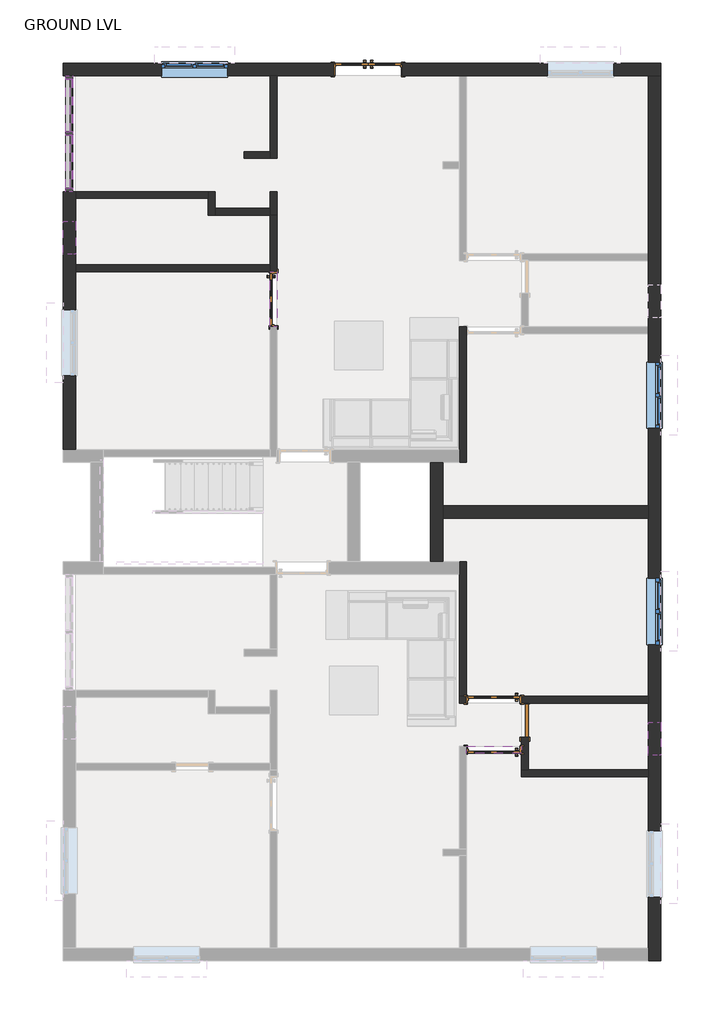
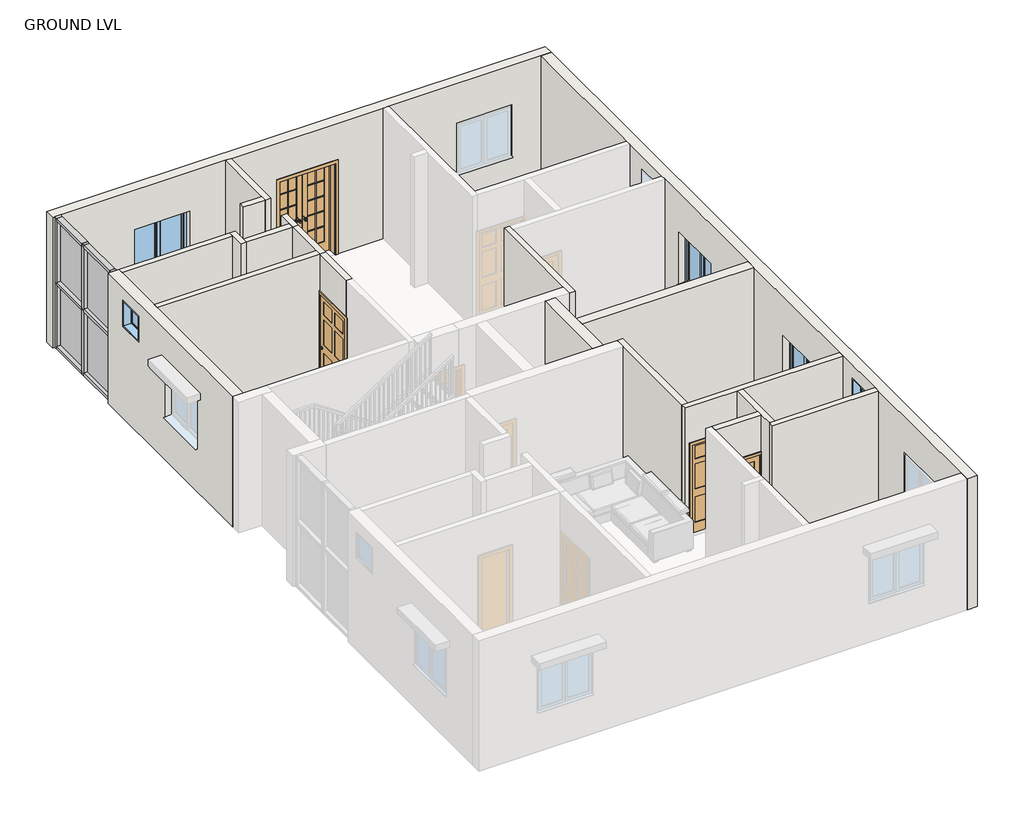
# One storey, part 2 of 4: 20 walls, 12 members, 5 doors, 5 windows, 4 plates.
"""IFC4 building model written with IfcOpenShell, lengths in millimetres."""

from ifc_helpers import new_model, si_unit, frame, origin, place, context, project, spatial, polyline, outline, extrude, faceted_brep, transform, mapped, element, save
from components import door_interior_double_full_glass_wood_4_x_7_exterior_door_6b6f14de, door_6a452240, door_3d68aebc, single_flush_flush_door_2_x_7_931cabab, member_801a2072, member_82905deb, member_88aa5c81, member_4491d118, system_panel_glazed_a8655be6, window_80340324, w2_windows_4_x_4_9dec5fc7

model = new_model("IFC4")

# Units and contexts
model_context = context("Model", 3, world=origin())
ifc_project = project(units=[si_unit("LENGTHUNIT", "METRE", prefix="MILLI")], contexts=[model_context])

# Site, building, storey
site = spatial("IfcSite", under=ifc_project)
building = spatial("IfcBuilding", under=site)
storey = spatial("IfcBuildingStorey", under=building, Name="GROUND LVL", Elevation=3048.0)

# Doors
placement = place(None, origin())
door_interior_double_full_glass_wood_4_x_7_exterior_door_shape = door_interior_double_full_glass_wood_4_x_7_exterior_door_6b6f14de(model_context)
element("IfcDoor", 1, ObjectType="Door-Interior-Double-Full Glass-Wood : 4' x 7' exterior door", at=placement, inside=storey, context=model_context, shape_type="MappedRepresentation", body=[
    mapped(door_interior_double_full_glass_wood_4_x_7_exterior_door_shape, transform((-817.6012202, 13160.1059003, 3048.0), x_axis=(1.0, 0.0, 0.0), y_axis=(0.0, 1.0, 0.0), z_axis=(0.0, 0.0, 1.0))),
])
door_shape = door_6a452240(model_context)
element("IfcDoor", 2, ObjectType="Door-Interior-Single-6_Panel-Wood : interior door 3' 4\" x 7'", at=placement, inside=storey, context=model_context, shape_type="MappedRepresentation", body=[
    mapped(door_shape, transform((-2560.6762202, 8927.8309003, 3048.0), x_axis=(0.0, -1.0, 0.0), y_axis=(1.0, 0.0, 0.0), z_axis=(0.0, 0.0, 1.0))),
])
element("IfcDoor", 3, ObjectType="Door-Interior-Single-6_Panel-Wood : interior door 3' 4\" x 7'", at=placement, inside=storey, context=model_context, shape_type="MappedRepresentation", body=[
    mapped(door_shape, transform((1493.7987798, 1565.0059003, 3048.0), x_axis=(-1.0, 0.0, 0.0), y_axis=(0.0, -1.0, 0.0), z_axis=(0.0, 0.0, 1.0))),
])
door_2_shape = door_3d68aebc(model_context)
element("IfcDoor", 4, ObjectType="Door-Interior-Single-6_Panel-Wood : interior door 3' 4\" x 7'", at=placement, inside=storey, context=model_context, shape_type="MappedRepresentation", body=[
    mapped(door_2_shape, transform((1493.7987798, 644.2559003, 3048.0), x_axis=(-1.0, 0.0, 0.0), y_axis=(0.0, -1.0, 0.0), z_axis=(0.0, 0.0, 1.0))),
])
single_flush_flush_door_2_x_7_shape = single_flush_flush_door_2_x_7_931cabab(model_context)
element("IfcDoor", 5, ObjectType="Single-Flush : flush door 2' x 7'", at=placement, inside=storey, context=model_context, shape_type="MappedRepresentation", body=[
    mapped(single_flush_flush_door_2_x_7_shape, transform((2065.2987798, 1180.8309003, 3048.0), x_axis=(0.0, 1.0, 0.0), y_axis=(-1.0, 0.0, 0.0), z_axis=(0.0, 0.0, 1.0))),
])

# Members
member_shape = member_801a2072(model_context)
element("IfcMember", 6, ObjectType="Rectangular Mullion : 2.5\" x 5\" rectangular", at=placement, inside=storey, context=model_context, shape_type="MappedRepresentation", body=[
    mapped(member_shape, transform((-6316.7012202, 10972.5309003, 6096.0), x_axis=(0.0, 0.0, 1.0), y_axis=(-1.0, 0.0, 0.0), z_axis=(0.0, -1.0, 0.0))),
])
element("IfcMember", 7, ObjectType="Rectangular Mullion : 2.5\" x 5\" rectangular", at=placement, inside=storey, context=model_context, shape_type="MappedRepresentation", body=[
    mapped(member_shape, transform((-6316.7012202, 12007.5809003, 6096.0), x_axis=(0.0, 0.0, 1.0), y_axis=(-1.0, 0.0, 0.0), z_axis=(0.0, -1.0, 0.0))),
])
element("IfcMember", 8, ObjectType="Rectangular Mullion : 2.5\" x 5\" rectangular", at=placement, inside=storey, context=model_context, shape_type="MappedRepresentation", body=[
    mapped(member_shape, transform((-6316.7012202, 12979.1309003, 3048.0), x_axis=(0.0, 0.0, -1.0), y_axis=(-1.0, 0.0, 0.0), z_axis=(0.0, 1.0, 0.0))),
])
element("IfcMember", 9, ObjectType="Rectangular Mullion : 2.5\" x 5\" rectangular", at=placement, inside=storey, context=model_context, shape_type="MappedRepresentation", body=[
    mapped(member_shape, transform((-6316.7012202, 11944.0809003, 3048.0), x_axis=(0.0, 0.0, -1.0), y_axis=(-1.0, 0.0, 0.0), z_axis=(0.0, 1.0, 0.0))),
])
member_2_shape = member_82905deb(model_context)
element("IfcMember", 10, ObjectType="Rectangular Mullion : 2.5\" x 5\" rectangular", at=placement, inside=storey, context=model_context, shape_type="MappedRepresentation", body=[
    mapped(member_2_shape, transform((-6316.7012202, 11975.8309003, 3048.0), x_axis=(0.0, -1.0, 0.0), y_axis=(-1.0, 0.0, 0.0), z_axis=(0.0, 0.0, -1.0))),
])
member_3_shape = member_88aa5c81(model_context)
element("IfcMember", 11, ObjectType="Rectangular Mullion : 2.5\" x 5\" rectangular", at=placement, inside=storey, context=model_context, shape_type="MappedRepresentation", body=[
    mapped(member_3_shape, transform((-6316.7012202, 12007.5809003, 4572.0), x_axis=(0.0, 0.0, 1.0), y_axis=(-1.0, 0.0, 0.0), z_axis=(0.0, -1.0, 0.0))),
])
element("IfcMember", 12, ObjectType="Rectangular Mullion : 2.5\" x 5\" rectangular", at=placement, inside=storey, context=model_context, shape_type="MappedRepresentation", body=[
    mapped(member_3_shape, transform((-6316.7012202, 10972.5309003, 4572.0), x_axis=(0.0, 0.0, 1.0), y_axis=(-1.0, 0.0, 0.0), z_axis=(0.0, -1.0, 0.0))),
])
element("IfcMember", 13, ObjectType="Rectangular Mullion : 2.5\" x 5\" rectangular", at=placement, inside=storey, context=model_context, shape_type="MappedRepresentation", body=[
    mapped(member_2_shape, transform((-6316.7012202, 11975.8309003, 4572.0), x_axis=(0.0, -1.0, 0.0), y_axis=(-1.0, 0.0, 0.0), z_axis=(0.0, 0.0, -1.0))),
])
member_4_shape = member_4491d118(model_context)
element("IfcMember", 14, ObjectType="Rectangular Mullion : 2.5\" x 5\" rectangular", at=placement, inside=storey, context=model_context, shape_type="MappedRepresentation", body=[
    mapped(member_4_shape, transform((-6316.7012202, 10909.0309003, 3048.0), x_axis=(0.0, -1.0, 0.0), y_axis=(-1.0, 0.0, 0.0), z_axis=(0.0, 0.0, -1.0))),
])
element("IfcMember", 15, ObjectType="Rectangular Mullion : 2.5\" x 5\" rectangular", at=placement, inside=storey, context=model_context, shape_type="MappedRepresentation", body=[
    mapped(member_4_shape, transform((-6316.7012202, 13042.6309003, 6096.0), x_axis=(0.0, 1.0, 0.0), y_axis=(-1.0, 0.0, 0.0), z_axis=(0.0, 0.0, 1.0))),
])
element("IfcMember", 16, ObjectType="Rectangular Mullion : 2.5\" x 5\" rectangular", at=placement, inside=storey, context=model_context, shape_type="MappedRepresentation", body=[
    mapped(member_4_shape, transform((-6316.7012202, 10909.0309003, 4572.0), x_axis=(0.0, -1.0, 0.0), y_axis=(-1.0, 0.0, 0.0), z_axis=(0.0, 0.0, -1.0))),
])
element("IfcMember", 17, ObjectType="Rectangular Mullion : 2.5\" x 5\" rectangular", at=placement, inside=storey, context=model_context, shape_type="MappedRepresentation", body=[
    mapped(member_4_shape, transform((-6316.7012202, 13042.6309003, 4572.0), x_axis=(0.0, 1.0, 0.0), y_axis=(-1.0, 0.0, 0.0), z_axis=(0.0, 0.0, 1.0))),
])

# Plates
system_panel_glazed_shape = system_panel_glazed_a8655be6(model_context)
element("IfcPlate", 18, ObjectType="System Panel : Glazed", at=placement, inside=storey, context=model_context, shape_type="MappedRepresentation", body=[
    mapped(system_panel_glazed_shape, transform((-6316.7012202, 12493.3559003, 3111.5), x_axis=(0.0, -1.0, 0.0), y_axis=(1.0, 0.0, 0.0), z_axis=(0.0, 0.0, 1.0))),
])
element("IfcPlate", 19, ObjectType="System Panel : Glazed", at=placement, inside=storey, context=model_context, shape_type="MappedRepresentation", body=[
    mapped(system_panel_glazed_shape, transform((-6316.7012202, 11458.3059003, 3111.5), x_axis=(0.0, -1.0, 0.0), y_axis=(1.0, 0.0, 0.0), z_axis=(0.0, 0.0, 1.0))),
])
element("IfcPlate", 20, ObjectType="System Panel : Glazed", at=placement, inside=storey, context=model_context, shape_type="MappedRepresentation", body=[
    mapped(system_panel_glazed_shape, transform((-6316.7012202, 12493.3559003, 4603.75), x_axis=(0.0, -1.0, 0.0), y_axis=(1.0, 0.0, 0.0), z_axis=(0.0, 0.0, 1.0))),
])
element("IfcPlate", 21, ObjectType="System Panel : Glazed", at=placement, inside=storey, context=model_context, shape_type="MappedRepresentation", body=[
    mapped(system_panel_glazed_shape, transform((-6316.7012202, 11458.3059003, 4603.75), x_axis=(0.0, -1.0, 0.0), y_axis=(1.0, 0.0, 0.0), z_axis=(0.0, 0.0, 1.0))),
])

# Walls
element("IfcWall", 22, ObjectType="OUTER WALL 9\"", at=placement, inside=storey, context=model_context, shape_type="Brep", body=[
    faceted_brep([(4567.1987798, 13042.6309003, 6096.0), (4338.5987798, 13042.6309003, 6096.0), (985.7987798, 13042.6309003, 6096.0), (858.7987798, 13042.6309003, 6096.0), (-2494.0012202, 13042.6309003, 6096.0), (-2621.0012202, 13042.6309003, 6096.0), (-6202.4012202, 13042.6309003, 6096.0), (-6431.0012202, 13042.6309003, 6096.0), (-6432.5887202, 13042.6309003, 6096.0), (-6432.5887202, 13042.6309003, 3048.0), (-6431.0012202, 13042.6309003, 3048.0), (-6202.4012202, 13042.6309003, 3048.0), (-2621.0012202, 13042.6309003, 3048.0), (-2494.0012202, 13042.6309003, 3048.0), (-1452.6012202, 13042.6309003, 3048.0), (-1452.6012202, 13042.6309003, 5207.0), (-182.6012202, 13042.6309003, 5207.0), (-182.6012202, 13042.6309003, 3048.0), (858.7987798, 13042.6309003, 3048.0), (985.7987798, 13042.6309003, 3048.0), (4338.5987798, 13042.6309003, 3048.0), (4567.1987798, 13042.6309003, 3048.0), (2479.7847416, 13042.6309003, 3962.4), (2479.7847416, 13042.6309003, 5181.6), (3698.9847416, 13042.6309003, 5181.6), (3698.9847416, 13042.6309003, 3962.4), (-3402.0512202, 13042.6309003, 3962.4), (-4621.2512202, 13042.6309003, 3962.4), (-4621.2512202, 13042.6309003, 5181.6), (-3402.0512202, 13042.6309003, 5181.6), (-6432.5887202, 13271.2309003, 6096.0), (4567.1987798, 13271.2309003, 6096.0), (4567.1987798, 13271.2309003, 3048.0), (-182.6012202, 13271.2309003, 3048.0), (-182.6012202, 13271.2309003, 5207.0), (-1452.6012202, 13271.2309003, 5207.0), (-1452.6012202, 13271.2309003, 3048.0), (-6432.5887202, 13271.2309003, 3048.0), (2479.7847416, 13271.2309003, 3962.4), (3698.9847416, 13271.2309003, 3962.4), (3698.9847416, 13271.2309003, 5181.6), (2479.7847416, 13271.2309003, 5181.6), (-3402.0512202, 13271.2309003, 3962.4), (-3402.0512202, 13271.2309003, 5181.6), (-4621.2512202, 13271.2309003, 5181.6), (-4621.2512202, 13271.2309003, 3962.4)], [[[0, 1, 2, 3, 4, 5, 6, 7, 8, 9, 10, 11, 12, 13, 14, 15, 16, 17, 18, 19, 20, 21], [22, 23, 24, 25], [26, 27, 28, 29]], [[30, 31, 32, 33, 34, 35, 36, 37], [38, 39, 40, 41], [42, 43, 44, 45]], [[9, 37, 36, 14, 13, 12, 11, 10]], [[32, 21, 20, 19, 18, 17, 33]], [[8, 7, 6, 5, 4, 3, 2, 1, 0, 31, 30]], [[9, 8, 30, 37]], [[0, 21, 32, 31]], [[16, 34, 33, 17]], [[34, 16, 15, 35]], [[35, 15, 14, 36]], [[23, 22, 38, 41]], [[24, 23, 41, 40]], [[25, 24, 40, 39]], [[22, 25, 39, 38]], [[43, 42, 26, 29]], [[44, 43, 29, 28]], [[45, 44, 28, 27]], [[42, 45, 27, 26]]]),
])
element("IfcWall", 23, ObjectType="OUTER WALL 9\"", at=placement, inside=storey, context=model_context, shape_type="Brep", body=[
    faceted_brep([(4338.5987798, 13042.6309003, 3048.0), (4338.5987798, 9766.0309003, 3048.0), (4338.5987798, 9639.0309003, 3048.0), (4338.5987798, 8419.8309003, 3048.0), (4338.5987798, 8292.8309003, 3048.0), (4338.5987798, 5130.5309003, 3048.0), (4338.5987798, 4901.9309003, 3048.0), (4338.5987798, 1625.3309003, 3048.0), (4338.5987798, 1498.3309003, 3048.0), (4338.5987798, 279.1309003, 3048.0), (4338.5987798, 152.1309003, 3048.0), (4338.5987798, -3010.1690997, 3048.0), (4338.5987798, -3238.7690997, 3048.0), (4338.5987798, -3238.7690997, 6096.0), (4338.5987798, -3010.1690997, 6096.0), (4338.5987798, 152.1309003, 6096.0), (4338.5987798, 279.1309003, 6096.0), (4338.5987798, 1498.3309003, 6096.0), (4338.5987798, 1625.3309003, 6096.0), (4338.5987798, 4901.9309003, 6096.0), (4338.5987798, 5130.5309003, 6096.0), (4338.5987798, 8292.8309003, 6096.0), (4338.5987798, 8419.8309003, 6096.0), (4338.5987798, 9639.0309003, 6096.0), (4338.5987798, 9766.0309003, 6096.0), (4338.5987798, 13042.6309003, 6096.0), (4338.5987798, 6552.9309003, 5181.6), (4338.5987798, 6552.9309003, 3962.4), (4338.5987798, 7772.1309003, 3962.4), (4338.5987798, 7772.1309003, 5181.6), (4338.5987798, 2577.8309003, 5181.6), (4338.5987798, 2577.8309003, 3962.4), (4338.5987798, 3797.0309003, 3962.4), (4338.5987798, 3797.0309003, 5181.6), (4338.5987798, 8584.9309003, 5791.2), (4338.5987798, 8584.9309003, 5181.6), (4338.5987798, 9194.5309003, 5181.6), (4338.5987798, 9194.5309003, 5791.2), (4338.5987798, 539.4809003, 5791.2), (4338.5987798, 539.4809003, 5181.6), (4338.5987798, 1149.0809003, 5181.6), (4338.5987798, 1149.0809003, 5791.2), (4338.5987798, -844.8190997, 4048.0), (4338.5987798, -844.8190997, 5267.2), (4338.5987798, -2064.0190997, 5267.2), (4338.5987798, -2064.0190997, 4048.0), (4567.1987798, -3238.7690997, 3048.0), (4567.1987798, 13042.6309003, 3048.0), (4567.1987798, 13042.6309003, 6096.0), (4567.1987798, -3238.7690997, 6096.0), (4567.1987798, 6552.9309003, 3962.4), (4567.1987798, 6552.9309003, 5181.6), (4567.1987798, 7772.1309003, 5181.6), (4567.1987798, 7772.1309003, 3962.4), (4567.1987798, 2577.8309003, 3962.4), (4567.1987798, 2577.8309003, 5181.6), (4567.1987798, 3797.0309003, 5181.6), (4567.1987798, 3797.0309003, 3962.4), (4567.1987798, 8584.9309003, 5181.6), (4567.1987798, 8584.9309003, 5791.2), (4567.1987798, 9194.5309003, 5791.2), (4567.1987798, 9194.5309003, 5181.6), (4567.1987798, 539.4809003, 5181.6), (4567.1987798, 539.4809003, 5791.2), (4567.1987798, 1149.0809003, 5791.2), (4567.1987798, 1149.0809003, 5181.6), (4567.1987798, -844.8190997, 5267.2), (4567.1987798, -844.8190997, 4048.0), (4567.1987798, -2064.0190997, 4048.0), (4567.1987798, -2064.0190997, 5267.2)], [[[0, 1, 2, 3, 4, 5, 6, 7, 8, 9, 10, 11, 12, 13, 14, 15, 16, 17, 18, 19, 20, 21, 22, 23, 24, 25], [26, 27, 28, 29], [30, 31, 32, 33], [34, 35, 36, 37], [38, 39, 40, 41], [42, 43, 44, 45]], [[46, 47, 48, 49], [50, 51, 52, 53], [54, 55, 56, 57], [58, 59, 60, 61], [62, 63, 64, 65], [66, 67, 68, 69]], [[12, 11, 10, 9, 8, 7, 6, 5, 4, 3, 2, 1, 0, 47, 46]], [[25, 24, 23, 22, 21, 20, 19, 18, 17, 16, 15, 14, 13, 49, 48]], [[0, 25, 48, 47]], [[13, 12, 46, 49]], [[51, 50, 27, 26]], [[52, 51, 26, 29]], [[53, 52, 29, 28]], [[50, 53, 28, 27]], [[55, 54, 31, 30]], [[56, 55, 30, 33]], [[57, 56, 33, 32]], [[54, 57, 32, 31]], [[34, 59, 58, 35]], [[35, 58, 61, 36]], [[36, 61, 60, 37]], [[59, 34, 37, 60]], [[38, 63, 62, 39]], [[39, 62, 65, 40]], [[64, 41, 40, 65]], [[63, 38, 41, 64]], [[43, 42, 67, 66]], [[44, 43, 66, 69]], [[45, 44, 69, 68]], [[42, 45, 68, 67]]]),
])
element("IfcWall", 24, ObjectType="OUTER WALL 9\"", at=placement, inside=storey, context=model_context, shape_type="Brep", body=[
    faceted_brep([(-6202.4012202, 6159.2309003, 6096.0), (-6202.4012202, 6159.2309003, 3048.0), (-6202.4012202, 9435.8309003, 3048.0), (-6202.4012202, 9562.8309003, 3048.0), (-6202.4012202, 10782.0309003, 3048.0), (-6202.4012202, 10909.0309003, 3048.0), (-6202.4012202, 10909.0309003, 6096.0), (-6202.4012202, 10782.0309003, 6096.0), (-6202.4012202, 9562.8309003, 6096.0), (-6202.4012202, 9435.8309003, 6096.0), (-6202.4012202, 9753.3309003, 5181.6), (-6202.4012202, 9753.3309003, 5791.2), (-6202.4012202, 10362.9309003, 5791.2), (-6202.4012202, 10362.9309003, 5181.6), (-6202.4012202, 7518.1309003, 4048.0), (-6202.4012202, 7518.1309003, 5267.2), (-6202.4012202, 8737.3309003, 5267.2), (-6202.4012202, 8737.3309003, 4048.0), (-6431.0012202, 6159.2309003, 3048.0), (-6431.0012202, 6159.2309003, 6096.0), (-6431.0012202, 10909.0309003, 6096.0), (-6431.0012202, 10909.0309003, 3048.0), (-6431.0012202, 9753.3309003, 5791.2), (-6431.0012202, 9753.3309003, 5181.6), (-6431.0012202, 10362.9309003, 5181.6), (-6431.0012202, 10362.9309003, 5791.2), (-6431.0012202, 7518.1309003, 4048.0), (-6431.0012202, 8737.3309003, 4048.0), (-6431.0012202, 8737.3309003, 5267.2), (-6431.0012202, 7518.1309003, 5267.2)], [[[0, 1, 2, 3, 4, 5, 6, 7, 8, 9], [10, 11, 12, 13], [14, 15, 16, 17]], [[18, 19, 20, 21], [22, 23, 24, 25], [26, 27, 28, 29]], [[1, 18, 21, 5, 4, 3, 2]], [[19, 0, 9, 8, 7, 6, 20]], [[1, 0, 19, 18]], [[22, 11, 10, 23]], [[23, 10, 13, 24]], [[12, 25, 24, 13]], [[11, 22, 25, 12]], [[6, 5, 21, 20]], [[15, 14, 26, 29]], [[16, 15, 29, 28]], [[17, 16, 28, 27]], [[14, 17, 27, 26]]]),
])
element("IfcWall", 25, ObjectType="OUTER WALL 9\"", at=placement, inside=storey, context=model_context, shape_type="Brep", body=[
    faceted_brep([(325.3987798, 5930.6309003, 3048.0), (325.3987798, 4101.8309003, 3048.0), (325.3987798, 4101.8309003, 6096.0), (325.3987798, 5930.6309003, 6096.0), (553.9987798, 5930.6309003, 3048.0), (553.9987798, 5930.6309003, 6096.0), (553.9987798, 5130.5309003, 6096.0), (553.9987798, 4901.9309003, 6096.0), (553.9987798, 4101.8309003, 6096.0), (553.9987798, 4101.8309003, 3048.0), (553.9987798, 4901.9309003, 3048.0), (553.9987798, 5130.5309003, 3048.0)], [[[0, 1, 2, 3]], [[4, 5, 6, 7, 8, 9, 10, 11]], [[1, 0, 4, 11, 10, 9]], [[3, 2, 8, 7, 6, 5]], [[2, 1, 9, 8]], [[0, 3, 5, 4]]]),
])
element("IfcWall", 26, ObjectType="OUTER WALL 9\"", at=placement, inside=storey, context=model_context, shape_type="SweptSolid", body=[
    extrude(outline(polyline([(4338.5987798, 4901.9309003), (553.9987798, 4901.9309003), (553.9987798, 5130.5309003), (4338.5987798, 5130.5309003), (4338.5987798, 4901.9309003)])), frame((0.0, 0.0, 3048.0), z_axis=(0.0, 0.0, 1.0), x_axis=(1.0, 0.0, 0.0)), (0.0, 0.0, 1.0), 3048.0),
])
element("IfcWall", 27, ObjectType="inner wall 5\"", at=placement, inside=storey, context=model_context, shape_type="Brep", body=[
    faceted_brep([(-2621.0012202, 13042.6309003, 3048.0), (-2621.0012202, 11645.6309003, 3048.0), (-2621.0012202, 11518.6309003, 3048.0), (-2621.0012202, 11518.6309003, 6096.0), (-2621.0012202, 11645.6309003, 6096.0), (-2621.0012202, 13042.6309003, 6096.0), (-2494.0012202, 13042.6309003, 3048.0), (-2494.0012202, 13042.6309003, 6096.0), (-2494.0012202, 11518.6309003, 6096.0), (-2494.0012202, 11518.6309003, 3048.0)], [[[0, 1, 2, 3, 4, 5]], [[6, 7, 8, 9]], [[2, 1, 0, 6, 9]], [[5, 4, 3, 8, 7]], [[0, 5, 7, 6]], [[3, 2, 9, 8]]]),
])
element("IfcWall", 28, ObjectType="inner wall 5\"", at=placement, inside=storey, context=model_context, shape_type="SweptSolid", body=[
    extrude(outline(polyline([(-3103.6012202, 11645.6309003), (-2621.0012202, 11645.6309003), (-2621.0012202, 11518.6309003), (-3103.6012202, 11518.6309003), (-3103.6012202, 11645.6309003)])), frame((0.0, 0.0, 3048.0), z_axis=(0.0, 0.0, 1.0), x_axis=(1.0, 0.0, 0.0)), (0.0, 0.0, 1.0), 3048.0),
])
element("IfcWall", 29, ObjectType="inner wall 5\"", at=placement, inside=storey, context=model_context, shape_type="SweptSolid", body=[
    extrude(outline(polyline([(-3764.0012202, 10782.0309003), (-6202.4012202, 10782.0309003), (-6202.4012202, 10909.0309003), (-3764.0012202, 10909.0309003), (-3764.0012202, 10782.0309003)])), frame((0.0, 0.0, 3048.0), z_axis=(0.0, 0.0, 1.0), x_axis=(1.0, 0.0, 0.0)), (0.0, 0.0, 1.0), 3048.0),
])
element("IfcWall", 30, ObjectType="inner wall 5\"", at=placement, inside=storey, context=model_context, shape_type="Brep", body=[
    faceted_brep([(-3764.0012202, 10909.0309003, 3048.0), (-3764.0012202, 10782.0309003, 3048.0), (-3764.0012202, 10477.2309003, 3048.0), (-3764.0012202, 10477.2309003, 6096.0), (-3764.0012202, 10782.0309003, 6096.0), (-3764.0012202, 10909.0309003, 6096.0), (-3637.0012202, 10909.0309003, 3048.0), (-3637.0012202, 10909.0309003, 6096.0), (-3637.0012202, 10604.2309003, 6096.0), (-3637.0012202, 10477.2309003, 6096.0), (-3637.0012202, 10477.2309003, 3048.0), (-3637.0012202, 10604.2309003, 3048.0)], [[[0, 1, 2, 3, 4, 5]], [[6, 7, 8, 9, 10, 11]], [[2, 1, 0, 6, 11, 10]], [[5, 4, 3, 9, 8, 7]], [[0, 5, 7, 6]], [[3, 2, 10, 9]]]),
])
element("IfcWall", 31, ObjectType="inner wall 5\"", at=placement, inside=storey, context=model_context, shape_type="SweptSolid", body=[
    extrude(outline(polyline([(-2621.0012202, 10477.2309003), (-3637.0012202, 10477.2309003), (-3637.0012202, 10604.2309003), (-2621.0012202, 10604.2309003), (-2621.0012202, 10477.2309003)])), frame((0.0, 0.0, 3048.0), z_axis=(0.0, 0.0, 1.0), x_axis=(1.0, 0.0, 0.0)), (0.0, 0.0, 1.0), 3048.0),
])
element("IfcWall", 32, ObjectType="inner wall 5\"", at=placement, inside=storey, context=model_context, shape_type="Brep", body=[
    faceted_brep([(-2494.0012202, 10477.2309003, 3048.0), (-2494.0012202, 10909.0309003, 3048.0), (-2494.0012202, 10909.0309003, 6096.0), (-2494.0012202, 10477.2309003, 6096.0), (-2621.0012202, 10477.2309003, 3048.0), (-2621.0012202, 10477.2309003, 6096.0), (-2621.0012202, 10604.2309003, 6096.0), (-2621.0012202, 10909.0309003, 6096.0), (-2621.0012202, 10909.0309003, 3048.0), (-2621.0012202, 10604.2309003, 3048.0)], [[[0, 1, 2, 3]], [[4, 5, 6, 7, 8, 9]], [[1, 0, 4, 9, 8]], [[2, 1, 8, 7]], [[3, 2, 7, 6, 5]], [[0, 3, 5, 4]]]),
])
element("IfcWall", 33, ObjectType="inner wall 5\"", at=placement, inside=storey, context=model_context, shape_type="Brep", body=[
    faceted_brep([(-2621.0012202, 10477.2309003, 3048.0), (-2621.0012202, 9562.8309003, 3048.0), (-2621.0012202, 9435.8309003, 3048.0), (-2621.0012202, 9435.8309003, 5207.0), (-2621.0012202, 9435.8309003, 6096.0), (-2621.0012202, 9562.8309003, 6096.0), (-2621.0012202, 10477.2309003, 6096.0), (-2494.0012202, 10477.2309003, 3048.0), (-2494.0012202, 10477.2309003, 6096.0), (-2494.0012202, 9435.8309003, 6096.0), (-2494.0012202, 9435.8309003, 5207.0), (-2494.0012202, 9435.8309003, 3048.0)], [[[0, 1, 2, 3, 4, 5, 6]], [[7, 8, 9, 10, 11]], [[2, 1, 0, 7, 11]], [[6, 5, 4, 9, 8]], [[0, 6, 8, 7]], [[4, 3, 2, 11, 10, 9]]]),
])
element("IfcWall", 34, ObjectType="inner wall 5\"", at=placement, inside=storey, context=model_context, shape_type="SweptSolid", body=[
    extrude(outline(polyline([(-6202.4012202, 9562.8309003), (-2621.0012202, 9562.8309003), (-2621.0012202, 9435.8309003), (-6202.4012202, 9435.8309003), (-6202.4012202, 9562.8309003)])), frame((0.0, 0.0, 3048.0), z_axis=(0.0, 0.0, 1.0), x_axis=(1.0, 0.0, 0.0)), (0.0, 0.0, 1.0), 3048.0),
])
element("IfcWall", 35, ObjectType="inner wall 5\"", at=placement, inside=storey, context=model_context, shape_type="Brep", body=[
    faceted_brep([(858.7987798, 8419.8309003, 3048.0), (858.7987798, 6159.2309003, 3048.0), (858.7987798, 5930.6309003, 3048.0), (858.7987798, 5930.6309003, 6096.0), (858.7987798, 6159.2309003, 6096.0), (858.7987798, 8419.8309003, 6096.0), (985.7987798, 8419.8309003, 3048.0), (985.7987798, 8419.8309003, 5207.0), (985.7987798, 8419.8309003, 6096.0), (985.7987798, 8292.8309003, 6096.0), (985.7987798, 5930.6309003, 6096.0), (985.7987798, 5930.6309003, 3048.0)], [[[0, 1, 2, 3, 4, 5]], [[6, 7, 8, 9, 10, 11]], [[2, 1, 0, 6, 11]], [[5, 4, 3, 10, 9, 8]], [[3, 2, 11, 10]], [[0, 5, 8, 7, 6]]]),
])
element("IfcWall", 36, ObjectType="inner wall 5\"", at=placement, inside=storey, context=model_context, shape_type="SweptSolid", body=[
    extrude(outline(polyline([(2001.7987798, 583.9309003), (985.7987798, 583.9309003), (985.7987798, 710.9309003), (2001.7987798, 710.9309003), (2001.7987798, 583.9309003)])), frame((0.0, 0.0, 5207.0), z_axis=(0.0, 0.0, 1.0), x_axis=(1.0, 0.0, 0.0)), (0.0, 0.0, 1.0), 889.0),
])
element("IfcWall", 37, ObjectType="inner wall 5\"", at=placement, inside=storey, context=model_context, shape_type="Brep", body=[
    faceted_brep([(858.7987798, 1625.3309003, 6096.0), (985.7987798, 1625.3309003, 6096.0), (4338.5987798, 1625.3309003, 6096.0), (4338.5987798, 1625.3309003, 3048.0), (2001.7987798, 1625.3309003, 3048.0), (2001.7987798, 1625.3309003, 5207.0), (985.7987798, 1625.3309003, 5207.0), (985.7987798, 1625.3309003, 3048.0), (858.7987798, 1625.3309003, 3048.0), (4338.5987798, 1498.3309003, 6096.0), (2128.7987798, 1498.3309003, 6096.0), (2001.7987798, 1498.3309003, 6096.0), (858.7987798, 1498.3309003, 6096.0), (858.7987798, 1498.3309003, 3048.0), (985.7987798, 1498.3309003, 3048.0), (985.7987798, 1498.3309003, 5207.0), (2001.7987798, 1498.3309003, 5207.0), (2001.7987798, 1498.3309003, 3048.0), (2128.7987798, 1498.3309003, 3048.0), (4338.5987798, 1498.3309003, 3048.0)], [[[0, 1, 2, 3, 4, 5, 6, 7, 8]], [[9, 10, 11, 12, 13, 14, 15, 16, 17, 18, 19]], [[3, 19, 18, 17, 4]], [[13, 8, 7, 14]], [[2, 1, 0, 12, 11, 10, 9]], [[3, 2, 9, 19]], [[0, 8, 13, 12]], [[6, 15, 14, 7]], [[15, 6, 5, 16]], [[16, 5, 4, 17]]]),
])
element("IfcWall", 38, ObjectType="inner wall 5\"", at=placement, inside=storey, context=model_context, shape_type="Brep", body=[
    faceted_brep([(985.7987798, 1625.3309003, 3048.0), (985.7987798, 4101.8309003, 3048.0), (985.7987798, 4101.8309003, 6096.0), (985.7987798, 1625.3309003, 6096.0), (858.7987798, 1625.3309003, 3048.0), (858.7987798, 1625.3309003, 6096.0), (858.7987798, 3873.2309003, 6096.0), (858.7987798, 4101.8309003, 6096.0), (858.7987798, 4101.8309003, 3048.0), (858.7987798, 3873.2309003, 3048.0)], [[[0, 1, 2, 3]], [[4, 5, 6, 7, 8, 9]], [[1, 0, 4, 9, 8]], [[3, 2, 7, 6, 5]], [[0, 3, 5, 4]], [[2, 1, 8, 7]]]),
])
element("IfcWall", 39, ObjectType="inner wall 5\"", at=placement, inside=storey, context=model_context, shape_type="SweptSolid", body=[
    extrude(outline(polyline([(-2494.0012202, 9435.8309003), (-2494.0012202, 8419.8309003), (-2621.0012202, 8419.8309003), (-2621.0012202, 9435.8309003), (-2494.0012202, 9435.8309003)])), frame((0.0, 0.0, 5207.0), z_axis=(0.0, 0.0, 1.0), x_axis=(1.0, 0.0, 0.0)), (0.0, 0.0, 1.0), 889.0),
])
element("IfcWall", 40, ObjectType="inner wall 5\"", at=placement, inside=storey, context=model_context, shape_type="Brep", body=[
    faceted_brep([(4338.5987798, 279.1309003, 3048.0), (2128.7987798, 279.1309003, 3048.0), (2001.7987798, 279.1309003, 3048.0), (2001.7987798, 279.1309003, 6096.0), (2128.7987798, 279.1309003, 6096.0), (4338.5987798, 279.1309003, 6096.0), (4338.5987798, 152.1309003, 3048.0), (4338.5987798, 152.1309003, 6096.0), (2001.7987798, 152.1309003, 6096.0), (2001.7987798, 152.1309003, 3048.0)], [[[0, 1, 2, 3, 4, 5]], [[6, 7, 8, 9]], [[2, 1, 0, 6, 9]], [[5, 4, 3, 8, 7]], [[0, 5, 7, 6]], [[3, 2, 9, 8]]]),
])
element("IfcWall", 41, ObjectType="inner wall 5\"", at=placement, inside=storey, context=model_context, shape_type="Brep", body=[
    faceted_brep([(2128.7987798, 1485.6309003, 5181.6), (2128.7987798, 1485.6309003, 3048.0), (2128.7987798, 1498.3309003, 3048.0), (2128.7987798, 1498.3309003, 6096.0), (2128.7987798, 279.1309003, 6096.0), (2128.7987798, 279.1309003, 3048.0), (2128.7987798, 876.0309003, 3048.0), (2128.7987798, 876.0309003, 5181.6), (2001.7987798, 1498.3309003, 3048.0), (2001.7987798, 1485.6309003, 3048.0), (2001.7987798, 1485.6309003, 5181.6), (2001.7987798, 876.0309003, 5181.6), (2001.7987798, 876.0309003, 3048.0), (2001.7987798, 279.1309003, 3048.0), (2001.7987798, 279.1309003, 6096.0), (2001.7987798, 583.9309003, 6096.0), (2001.7987798, 710.9309003, 6096.0), (2001.7987798, 1498.3309003, 6096.0), (2001.7987798, 1498.3309003, 5207.0)], [[[0, 1, 2, 3, 4, 5, 6, 7]], [[8, 9, 10, 11, 12, 13, 14, 15, 16, 17, 18]], [[6, 5, 13, 12]], [[2, 1, 9, 8]], [[4, 3, 17, 16, 15, 14]], [[5, 4, 14, 13]], [[3, 2, 8, 18, 17]], [[10, 9, 1, 0]], [[11, 10, 0, 7]], [[12, 11, 7, 6]]]),
])

# Windows
window_shape = window_80340324(model_context)
element("IfcWindow", 42, ObjectType="Fixed : 24\" x 24\"", at=placement, inside=storey, context=model_context, shape_type="MappedRepresentation", body=[
    mapped(window_shape, transform((4452.8987798, 806.1809003, 4267.2), x_axis=(0.0, -1.0, 0.0), y_axis=(1.0, 0.0, 0.0), z_axis=(0.0, 0.0, 1.0))),
])
element("IfcWindow", 43, ObjectType="Fixed : 24\" x 24\"", at=placement, inside=storey, context=model_context, shape_type="MappedRepresentation", body=[
    mapped(window_shape, transform((-6316.7012202, 10020.0309003, 4267.2), x_axis=(0.0, -1.0, 0.0), y_axis=(1.0, 0.0, 0.0), z_axis=(0.0, 0.0, 1.0))),
])
w2_windows_4_x_4_shape = w2_windows_4_x_4_9dec5fc7(model_context)
element("IfcWindow", 44, ObjectType="w2 : windows 4' x 4'", at=placement, inside=storey, context=model_context, shape_type="MappedRepresentation", body=[
    mapped(w2_windows_4_x_4_shape, transform((-4011.6512202, 13156.9309003, 2962.4), x_axis=(-1.0, 0.0, 0.0), y_axis=(0.0, -1.0, 0.0), z_axis=(0.0, 0.0, 1.0))),
])
element("IfcWindow", 45, ObjectType="w2 : windows 4' x 4'", at=placement, inside=storey, context=model_context, shape_type="MappedRepresentation", body=[
    mapped(w2_windows_4_x_4_shape, transform((4452.8987798, 7162.5309003, 2962.4), x_axis=(0.0, 1.0, 0.0), y_axis=(-1.0, 0.0, 0.0), z_axis=(0.0, 0.0, 1.0))),
])
element("IfcWindow", 46, ObjectType="w2 : windows 4' x 4'", at=placement, inside=storey, context=model_context, shape_type="MappedRepresentation", body=[
    mapped(w2_windows_4_x_4_shape, transform((4452.8987798, 3187.4309003, 2962.4), x_axis=(0.0, 1.0, 0.0), y_axis=(-1.0, 0.0, 0.0), z_axis=(0.0, 0.0, 1.0))),
])

save(model, "model.ifc")

# Revit data of these elements
# Type "Door-Interior-Double-Full Glass-Wood : 4' x 7' exterior door"
#   Type Mark = "9"
#   Assembly Code = "C1020300"
#   Analytic Construction = "French door, wood frame with single glass"
#   Top Rail = 0' - 4 11/16"
#   Thickness = 0' - 1 3/8"
#   Thermal Resistance (R) = 1.0696 (h·ft²·°F)/BTU
#   Swing Angle [instance default] = 90.00°
#   Stiles = 0' - 4 3/4"
#   Rough Width = 4' - 2"
#   Rough Height = 7' - 1"
#   Panel Width = 2' - 0"
#   Height = 7' - 0"
#   Width = 4' - 0"
#   Heat Transfer Coefficient (U) = 0.9350 BTU/(h·ft²·°F)
#   Bottom Rail = 0' - 9 1/8"
#   Show Grill [instance default] = yes
#   Trim Material = Cherry
#   Panel Material = Cherry
#   Frame Material = Cherry
#   Door Handle Material = Aluminum
#   Visual Light Transmittance = 0
#   Solar Heat Gain Coefficient = 0
#   Wall Closure = (empty or 0)
#   Function = (empty or 0)
# Type "Door-Interior-Single-6_Panel-Wood : interior door 3' 4\" x 7'"
#   Type Mark = "11"
#   Assembly Code = "C1020300"
#   Analytic Construction = "Wooden"
#   Top Rail = 0' - 4 11/16"
#   Top Panel = 1' - 0"
#   Thickness = 0' - 1 3/8"
#   Thermal Resistance (R) = 2.5876 (h·ft²·°F)/BTU
#   Swing Angle [instance default] = 90.00°
#   Stiles = 0' - 4 3/4"
#   Rough Width = 3' - 4"
#   Rough Height = 7' - 1"
#   Mullion = 0' - 4 1/2"
#   Lock Rail = 0' - 7 1/2"
#   Intermediate Rail = 0' - 4 1/2"
#   Height = 7' - 0"
#   Width = 3' - 2"
#   Heat Transfer Coefficient (U) = 0.3865 BTU/(h·ft²·°F)
#   Bottom Rail = 0' - 9 1/8"
#   Trim Material = Cherry
#   Panel Material = Cherry
#   Frame Material = Cherry
#   Door Handle Material = Aluminum
#   Visual Light Transmittance = 0
#   Solar Heat Gain Coefficient = 0
#   Wall Closure = (empty or 0)
#   Function = (empty or 0)
# Type "Single-Flush : flush door 2' x 7'"
#   Type Mark = "12"
#   Construction Type Id = "MDOOR"
#   Assembly Code = "C1020"
#   Analytic Construction = "Metal"
#   Thickness = 0' - 2"
#   Heat Transfer Coefficient (U) = 0.651978 BTU/(h·ft²·°F)
#   Height = 7' - 0"
#   Trim Projection Ext = 0' - 1"
#   Trim Projection Int = 0' - 1"
#   Trim Width = 0' - 3"
#   Width = 2' - 0"
#   Define Thermal Properties by = 1
#   Door Material = Door - Panel
#   Frame Material = Door - Frame
#   Visual Light Transmittance = 0
#   Solar Heat Gain Coefficient = 0
#   Function = (empty or 0)
#   Wall Closure = (empty or 0)
# Type "Rectangular Mullion : 2.5\" x 5\" rectangular"
#   built-in parameter 1007304 = 0.416667 (stored number, unit not read)
#   built-in parameter 1007301 = 0.104167 (stored number, unit not read)
#   built-in parameter 1007300 = 0.104167 (stored number, unit not read)
# Type "System Panel : Glazed"
#   Construction Type Id = "GSP4R"
#   Analytic Construction = "1/8 in Pilkington single glazing"
#   Visual Light Transmittance = 0.9
#   Solar Heat Gain Coefficient = 0.86
#   Heat Transfer Coefficient (U) = 1.18115 BTU/(h·ft²·°F)
#   Define Thermal Properties by = 1
# Type "OUTER WALL 9\""
#   Assembly Code = "B2010"
#   Layers, outside or top first: 0' - 9" "ROSE COLOUR" (function 1)
# Type "inner wall 5\""
#   Assembly Code = "B2010"
#   Layers, outside or top first: 0' - 5" "ROSE COLOUR" (function 1)
# Type "Fixed : 24\" x 24\""
#   Type Mark = "3"
#   Construction Type Id = "GSP4R"
#   Assembly Code = "B2020100"
#   Analytic Construction = "1/8 in Pilkington single glazing"
#   Visual Light Transmittance = 0.9
#   Solar Heat Gain Coefficient = 0.78
#   Heat Transfer Coefficient (U) = 0.6496 BTU/(h·ft²·°F)
#   Height = 2' - 0"
#   Default Sill Height = 3' - 0"
#   Width = 2' - 0"
#   Window Inset = 0' - 0 3/4"
#   Define Thermal Properties by = 1
#   Define Thermal Properties by = 1
#   Glass Pane Material = Glass
#   Sash Material = Sash
#   Wall Closure = (empty or 0)
# Type "w2 : windows 4' x 4'"
#   Type Mark = "31"
#   Operation = "DoublePanelVertical"
#   Keynote = "16.05.01"
#   Analytic Construction = "<None>"
#   Rough Width = 4' - 0"
#   Rough Height = 4' - 0"
#   Rahmentiefe = 0' - 2.3622"
#   Rahmenhöhe unten = 0' - 3.14961"
#   Rahmehöhe oben = 0' - 3.14961"
#   Rahmenbreite = 0' - 2.3622"
#   Heat Transfer Coefficient (U) = 2.81836 BTU/(h·ft²·°F)
#   Height = 4' - 0"
#   Flügeltiefe = 0' - 2.3622"
#   Flügelbreite = 0' - 2.3622"
#   Einbautiefe (von außen) [instance default] = 0' - 5.51181"
#   Width = 4' - 0"
#   Kippflügel [instance default] = yes
#   Drehflügel im Grundriß darstellen [instance default] = no
#   Drehflügel [instance default] = yes
#   Define Thermal Properties by = 1
#   Rahmen [instance default] = none
#   Glas [instance default] = blue glass
#   Flügel [instance default] = WINDOW COLOUR WHITE
#   Fensterbank aussen [instance default] = WINDOW COLOUR WHITE
#   Fensterbank innen [instance default] = WINDOW COLOUR WHITE
#   Visual Light Transmittance = 0
#   Thermal Resistance (R) = 0
#   Solar Heat Gain Coefficient = 0
#   Wall Closure = (empty or 0)
# Element 1 (IfcDoor, "Door-Interior-Double-Full Glass-Wood : 4' x 7' exterior door")
#   Swing Angle = 90.00°
#   Show Grill = yes
#   Phase Created = New Construction
#   Materials on its faces: "Cherry", "Aluminum", "Glass"
# Elements 2, 3, 4 (IfcDoor, "Door-Interior-Single-6_Panel-Wood : interior door 3' 4\" x 7'")
#   Swing Angle = 90.00°
#   Phase Created = New Construction
#   Materials on its faces: "Cherry", "Aluminum"
# Element 5 (IfcDoor, "Single-Flush : flush door 2' x 7'")
#   Phase Created = New Construction
#   Materials on its faces: "Door - Frame", "Door - Panel"
# Elements 6, 7, 8, 9, 10, 11, 12, 13, 14, 15, 16, 17 (IfcMember, "Rectangular Mullion : 2.5\" x 5\" rectangular")
#   Phase Created = New Construction
#   Materials on its faces: "Aluminum"
# Elements 18, 19, 20, 21 (IfcPlate, "System Panel : Glazed")
#   Phase Created = New Construction
#   Materials on its faces: "Glass"
# Elements 22, 23, 24, 25, 26 (IfcWall, "OUTER WALL 9\"")
#   Top Offset = 0' - 0"
#   Base Offset = 0' - 0"
#   wall height = 10' - 0"
#   Phase Created = New Construction
#   Base Constraint = GROUND LVL
#   Top Constraint = 1 ST FLOOR
#   Materials on its faces: "ROSE COLOUR"
# Elements 27, 28, 29, 30, 31, 32, 33, 34, 35, 36, 37, 38, 39, 40, 41 (IfcWall, "inner wall 5\"")
#   Top Offset = 0' - 0"
#   Base Offset = 0' - 0"
#   wall height = 10' - 0"
#   Phase Created = New Construction
#   Base Constraint = GROUND LVL
#   Top Constraint = 1 ST FLOOR
#   Materials on its faces: "ROSE COLOUR"
# Element 42 (IfcWindow, "Fixed : 24\" x 24\"")
#   Mark = "15"
#   Phase Created = New Construction
#   Materials on its faces: "Sash", "Glass"
# Element 43 (IfcWindow, "Fixed : 24\" x 24\"")
#   Mark = "16"
#   Phase Created = New Construction
#   Materials on its faces: "Sash", "Glass"
# Element 44 (IfcWindow, "w2 : windows 4' x 4'")
#   Mark = "8"
#   Phase Created = New Construction
#   Materials on its faces: "WINDOW COLOUR WHITE", "blue glass"
# Element 45 (IfcWindow, "w2 : windows 4' x 4'")
#   Mark = "11"
#   Phase Created = New Construction
#   Materials on its faces: "WINDOW COLOUR WHITE", "blue glass"
# Element 46 (IfcWindow, "w2 : windows 4' x 4'")
#   Mark = "12"
#   Phase Created = New Construction
#   Materials on its faces: "WINDOW COLOUR WHITE", "blue glass"
# Materials
#   "Cherry": class "Wood", colour RGB 226 177 128, transparency 0, Description = "Prunus Serotina", Cost = 0
#   "Aluminum": class "Metal", colour RGB 247 247 247, transparency 0, Description = "Aluminum 6061", Cost = 0
#   "Door - Panel": class "Wood", colour RGB 210 159 95, transparency 0, Cost = 0
#   "Door - Frame": colour RGB 118 70 51, transparency 0, Cost = 0
#   "ROSE COLOUR": class "Generic", colour RGB 120 120 120, transparency 0, Cost = 0
#   "Glass": class "Glass", colour RGB 0 128 192, transparency 0.75, Description = "Soda Lime Glass", Cost = 0
#   "Sash": class "Wood", colour RGB 224 178 126, transparency 0, Cost = 0
#   "blue glass": class "System", colour RGB 0 0 255, transparency 0.75, Cost = 0
#   "WINDOW COLOUR WHITE": class "Generic", colour RGB 120 120 120, transparency 0, Cost = 0
